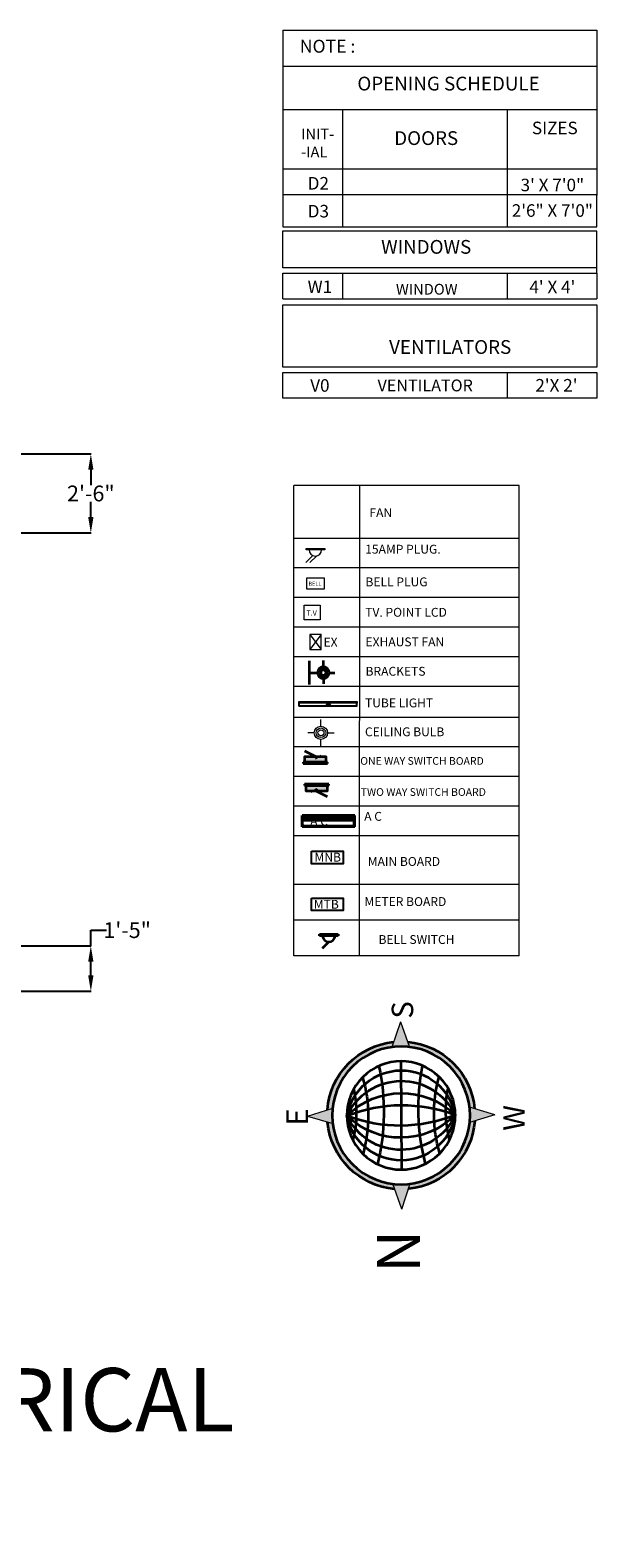
# Model space of a CAD drawing. Units: inches. Extents: x 329 to 1300, y 173 to 760.
# Tile 3 of 3: x 1085 to 1300, y 173 to 746. Entities that reach past the tile are written whole.
import ezdxf

# ---------------------------------------------------------------- set-up
doc = ezdxf.new("R2010")
doc.units = ezdxf.units.IN
doc.header["$MEASUREMENT"] = 0
doc.linetypes.add('HIDDEN', pattern=[0.375, 0.25, -0.125])
for name, color, linetype, lineweight in [('A -Elec', 6, 'Continuous', 18), ('A- WALL', 7, 'Continuous', 35), ('A-ANNO-SCHD', 80, 'Continuous', 13), ('A-ANNO-SCHD-HIDN', 80, 'HIDDEN', 13), ('A-ANNO-SYMB', 7, 'Continuous', 18), ('A-ANNO-TITL', 1, 'Continuous', 25), ('A-TEXT', 7, 'Continuous', 9), ('DIM', 7, 'Continuous', 9), ('DIMENSION', 80, 'Continuous', 13), ('E-ANNO-LEGD', 7, 'Continuous', 13), ('E-COMM', 1, 'Continuous', 18), ('E-EQPM-FANS', 1, 'Continuous', 18), ('E-LITE', 6, 'Continuous', 18), ('E-LITE-SWCH', 1, 'Continuous', 18), ('E-POWR-DEVC', 1, 'Continuous', 18), ('E-POWR-PANL', 1, 'Continuous', 25), ('Elec', 1, 'Continuous', 35), ('M-HVAC-EQPM', 1, 'Continuous', 18)]:
    doc.layers.add(name, color=color, linetype=linetype, lineweight=lineweight)
doc.styles.get("Standard").update_dxf_attribs({"font": 'arial.ttf'})
doc.dimstyles.get("Standard").update_dxf_attribs({"dimtxt": 6, "dimasz": 6, "dimexe": 0.18, "dimexo": 0.0625, "dimgap": 0.09, "dimtad": 0, "dimtih": 1, "dimtoh": 1, "dimdec": 1, "dimzin": 0, "dimdsep": 46, "dimlunit": 3, "dimtxsty": 'Standard', "dimcen": 0.09, "dimadec": 0, "dimazin": 0, "dimtfac": 1, "dimtdec": 1, "dimtofl": 0, "dimtmove": 0, "dimatfit": 3, "dimfxl": 1, "dimtolj": 1, "dimtzin": 0, "dimarcsym": 0})

# ---------------------------------------------------------------- blocks, each defined once
blk = doc.blocks.new('BELL SWITCH')
at = {"layer": 'Elec'}
for p, q in [((4981.810695824261, 3401.308516663301), (4981.810695824261, 3402.267205949833)), ((4981.810695824261, 3402.267205949833), (4993.567325880143, 3402.267205949833)), ((4993.567325880143, 3401.308516663301), (4981.810695824261, 3401.308516663301)), ((4987.689010852202, 3397.361748155474), (4983.521874140887, 3393.30038126191)), ((4993.567325880143, 3402.267205949833), (4993.567325880143, 3401.308516663301))]:
    blk.add_line(p, q, dxfattribs=at)
blk.add_arc((4987.689010852202, 3401.308516663301), 3.946768507828181, 180, 0, dxfattribs=at)
blk = doc.blocks.new('splight')
at = {"layer": 'Elec'}
for p, q in [((4618.165493646445, 527.1595508907546), (4627.57380882646, 527.1595508907546)), ((4622.869651236451, 527.1595508907546), (4622.869651236451, 523.8688723625129)), ((4620.576181531769, 521.5754026578305), (4618.052205676129, 521.5754026578305)), ((4622.869651236451, 519.2819329531479), (4622.869651236451, 517.0346704452847)), ((4625.163120941137, 521.5754026578305), (4627.232633020232, 521.5754026578305))]:
    blk.add_line(p, q, dxfattribs=at)
for radius in [2.293469704682637, 1.668469704682639, 1.043469704682639]:
    blk.add_circle((4622.869651236451, 521.5754026578305), radius, dxfattribs=at)
blk = doc.blocks.new('CIELING')
at = {"layer": 'A -Elec'}
for p, q in [((1070.869500591183, -8395.655580837194), (1070.869500591183, -8391.485789029257)), ((1066.613971407157, -8399.911110021205), (1062.44417959922, -8399.911110021205)), ((1070.869500591183, -8408.33643101315), (1070.869500591183, -8404.166639205214)), ((1075.125029775208, -8399.911110021205), (1079.294821583145, -8399.911110021205))]:
    blk.add_line(p, q, dxfattribs=at)
for radius in [4.255529184009533, 3.095842734009534, 1.936156284009533]:
    blk.add_circle((1070.869500591183, -8399.911110021205), radius, dxfattribs=at)
blk = doc.blocks.new('tube')
at = {"layer": 'A -Elec'}
for p, q in [((4592.607752765609, 556.7543292074987), (4641.607752765609, 556.7543292074987)), ((4592.607752765609, 555.2543292074988), (4592.607752765609, 556.7543292074987)), ((4593.107752765609, 555.2543292074988), (4593.107752765609, 556.7543292074987)), ((4593.107752765609, 556.3299144522243), (4593.407752765609, 556.3299144522243)), ((4593.107752765609, 556.2104979518087), (4593.407752765609, 556.2104979518087)), ((4593.107752765609, 555.8060867251079), (4593.407752765609, 555.8060867251079)), ((4593.107752765609, 555.6866702246923), (4593.407752765609, 555.6866702246923)), ((4593.407752765609, 555.2543292074988), (4593.407752765609, 556.7543292074987)), ((4593.407752765609, 556.5043292074988), (4640.807752765609, 556.5043292074988)), ((4593.407752765609, 556.2543292074987), (4640.807752765609, 556.2543292074987)), ((4593.407752765609, 556.0043292074988), (4640.807752765609, 556.0043292074988)), ((4593.407752765609, 555.7543292074988), (4640.807752765609, 555.7543292074988)), ((4593.407752765609, 555.5043292074988), (4640.807752765609, 555.5043292074988)), ((4640.807752765609, 555.2543292074988), (4640.807752765609, 556.7543292074987)), ((4640.807752765609, 556.3299144522243), (4641.107752765608, 556.3299144522243)), ((4640.807752765609, 556.2104979518087), (4641.107752765608, 556.2104979518087)), ((4640.807752765609, 555.8060867251079), (4641.107752765608, 555.8060867251079)), ((4640.807752765609, 555.6866702246923), (4641.107752765608, 555.6866702246923)), ((4641.107752765608, 556.7543292074987), (4641.107752765608, 555.2543292074988)), ((4641.107752765608, 555.2543292074988), (4641.107752765608, 556.7543292074987)), ((4641.607752765609, 556.7543292074987), (4641.607752765609, 555.2543292074988)), ((4592.607752765609, 552.7543292074987), (4592.607752765609, 555.2543292074988)), ((4592.607752765609, 552.7543292074987), (4641.607752765609, 552.7543292074987)), ((4641.107752765608, 555.2543292074988), (4593.107752765609, 555.2543292074988)), ((4593.107752765609, 555.2543292074988), (4593.107752765609, 553.2543292074988)), ((4593.107752765609, 553.2543292074988), (4593.107752765609, 555.2543292074988)), ((4593.107752765609, 553.2543292074988), (4641.607752765609, 553.2543292074988)), ((4641.107752765608, 553.2543292074988), (4641.107752765608, 555.2543292074988)), ((4641.607752765609, 552.7543292074987), (4641.607752765609, 555.2543292074988))]:
    blk.add_line(p, q, dxfattribs=at)
for points in [[(4615.603450108063, 553.2543292074988), (4619.112055423154, 553.2543292074988), (4619.112055423154, 554.3062122222327), (4615.603450108063, 554.3062122222327)], [(4619.112055423154, 553.7802707148657), (4619.112055423154, 553.7802707148657), (4619.112055423154, 553.7802707148657), (4619.112055423154, 553.7802707148657)], [(4619.112055423154, 553.7802707148657), (4619.813791770798, 553.7802707148657), (4619.813791770798, 553.2543292074988), (4619.112055423154, 553.2543292074988)]]:
    blk.add_lwpolyline(points, close=True, dxfattribs=at)
blk = doc.blocks.new('ac')
at = {"layer": 'Elec'}
for p, q in [((12718.33512872629, -53.78451556294852), (12674.35721837807, -53.78451556294852)), ((12674.35721837806, -63.01930683579224), (12674.35721837807, -53.78451556294852)), ((12674.88506837807, -57.52248662285011), (12717.80727872628, -57.52248662285011)), ((12675.81311487755, -57.52248662285011), (12675.81311487755, -53.78451556294851)), ((12717.02869991749, -54.85019267976269), (12675.81311487755, -54.85019267976269)), ((12717.02869991749, -56.20859049643797), (12675.81311487755, -56.20859049643797)), ((12717.02869991748, -57.52248662285011), (12717.02869991749, -53.78451556294851)), ((12718.33512872629, -63.01930683579224), (12718.33512872629, -53.78451556294852)), ((12718.33512872629, -63.01930683579224), (12674.35721837806, -63.01930683579224))]:
    blk.add_line(p, q, dxfattribs=at)
at = {"layer": 'Elec', "ltscale": 0.1}
for p, q in [((12674.88506837807, -61.49145683579366), (12674.88506837807, -53.78451556294851)), ((12717.02869991749, -54.35872395628861), (12675.81311487755, -54.35872395628861)), ((12717.02869991749, -55.65507023101156), (12675.81311487755, -55.65507023101157)), ((12717.02869991749, -56.84485043173038), (12675.81311487755, -56.84485043173037)), ((12716.80727872628, -62.49145683579365), (12675.88506837807, -62.49145683579365)), ((12717.80727872628, -61.49145683579366), (12717.80727872628, -53.78451556294851))]:
    blk.add_line(p, q, dxfattribs=at)
at = {"layer": 'Elec'}
for centre, start, end in [((12675.88506837807, -61.49145683579366), 180, 270), ((12716.80727872628, -61.49145683579366), 270, 0)]:
    blk.add_arc(centre, 1, start, end, dxfattribs=at)
blk = doc.blocks.new('DIRECTION')
at = {"layer": 'DIM', "ltscale": 35}
h = blk.add_hatch(color=256, dxfattribs=at)
h.dxf.hatch_style = 1
edge = h.paths.add_edge_path()
edge.add_line((2597.24832190935, 2408.269559539512), (2601.856533232682, 2393.62299110183))
edge.add_ellipse((2597.639423319343, 2353.481842285464), major_axis=(28.54028595385228, -28.5402859538523), ratio=0.9999999999827393, start_angle=129.0026750704451, end_angle=135.4089982327699)
edge.add_ellipse((2597.639423319602, 2353.481842285464), major_axis=(-28.54028595291803, -28.54028595291801), ratio=0.999999999985297, start_angle=225.4089982331304, end_angle=231.8159173823239)
edge.add_line((2592.849261358955, 2393.558645959323), (2597.248321909339, 2408.269559539583))
h = blk.add_hatch(color=256, dxfattribs=at)
h.dxf.hatch_style = 1
edge = h.paths.add_edge_path()
edge.add_line((2637.716337406115, 2348.692604170624), (2640.725786551334, 2349.752367405582))
edge.add_ellipse((2597.639423319343, 2353.481842285464), major_axis=(-30.58057945317442, -30.5805794531744), ratio=0.9999999999976388, start_angle=50.166226554127775, end_angle=130.0529151095595, ccw=False)
edge.add_line((2601.533664809112, 2310.41005845266), (2602.42916840349, 2313.404988786752))
edge.add_ellipse((2597.639423319343, 2353.481842285464), major_axis=(-28.54028595136435, -28.54028595136432), ratio=0.9999999999994514, start_angle=51.81532139532596, end_angle=128.185403391547)
edge = h.paths.add_edge_path()
edge.add_line((2593.421895860988, 2313.340737337358), (2594.360152675466, 2310.358877830749))
edge.add_ellipse((2597.639423319343, 2353.481842285464), major_axis=(-30.58057945314276, -30.58057945314273), ratio=0.9999999999967295, start_angle=320.7650813562228, end_angle=400.6513322142664, ccw=False)
edge.add_line((2554.610693956437, 2349.137635932355), (2557.634965847779, 2348.12094433685))
edge.add_ellipse((2597.639423319343, 2353.481842285464), major_axis=(28.54028595137265, -28.54028595137269), ratio=0.9999999999998977, start_angle=232.6325930742551, end_angle=309.0020790836279)
edge = h.paths.add_edge_path()
edge.add_line((2557.562509232831, 2358.271080400352), (2554.553060087694, 2357.211317165394))
edge.add_ellipse((2597.639423319343, 2353.481842285464), major_axis=(-30.58057945310715, -30.58057945310715), ratio=0.9999999999999497, start_angle=230.1666642515818, end_angle=310.0529151095499, ccw=False)
edge.add_line((2593.744852793148, 2396.553596367937), (2592.849261358943, 2393.558645959394))
edge.add_ellipse((2597.639423319343, 2353.481842285464), major_axis=(28.5402859513619, -28.54028595136188), ratio=0.9999999999987931, start_angle=141.8159173820852, end_angle=218.1854033915469)
edge = h.paths.add_edge_path()
edge.add_line((2601.85653323267, 2393.622991101876), (2600.918364535997, 2396.604831790109))
edge.add_ellipse((2597.639423319343, 2353.481842285464), major_axis=(-30.58057945312165, -30.58057945312163), ratio=0.9999999999985156, start_angle=140.765081356223, end_angle=220.6517699116423, ccw=False)
edge.add_line((2640.668152682508, 2357.826048638621), (2637.643880791167, 2358.842740234127))
edge.add_ellipse((2597.639423319343, 2353.481842285464), major_axis=(28.54028595137743, -28.54028595137745), ratio=0.9999999999999049, start_angle=52.63259307425506, end_angle=129.0026750705646)
h = blk.add_hatch(color=256, dxfattribs=at)
h.dxf.hatch_style = 1
edge = h.paths.add_edge_path()
edge.add_ellipse((2597.639423319343, 2353.481842285464), major_axis=(-28.54028595210723, -28.54028595210721), ratio=0.999999999994473, start_angle=308.1854033915466, end_angle=322.6325930742547)
edge.add_line((2557.634965847779, 2348.120944336826), (2542.851706063651, 2353.090740875343))
edge.add_line((2542.851706063651, 2353.090740875343), (2557.562509232831, 2358.271080400328))
h = blk.add_hatch(color=256, dxfattribs=at)
h.dxf.hatch_style = 1
edge = h.paths.add_edge_path()
edge.add_line((2637.643880791167, 2358.84274023415), (2652.427140575295, 2353.87294369554))
edge.add_line((2652.427140575295, 2353.87294369554), (2637.716337406114, 2348.692604170648))
edge.add_ellipse((2597.639423319343, 2353.481842285464), major_axis=(-28.54028595030189, -28.54028595030183), ratio=0.9999999999925798, start_angle=128.1854033915468, end_angle=142.632593074255)
h = blk.add_hatch(color=256, dxfattribs=at)
h.dxf.hatch_style = 1
edge = h.paths.add_edge_path()
edge.add_line((2602.42916840349, 2313.404988786869), (2598.030524729594, 2298.694125031464))
edge.add_line((2598.030524729594, 2298.69412503137), (2593.421895860988, 2313.340737337334))
edge.add_ellipse((2597.639423319602, 2353.481842285464), major_axis=(28.54028595190623, -28.54028595190623), ratio=0.9999999999939888, start_angle=-50.99792091661058, end_angle=-44.59100176735014)
edge.add_ellipse((2597.639423319343, 2353.481842285464), major_axis=(-28.54028595335771, -28.54028595335769), ratio=0.9999999999832972, start_angle=45.40899823301023, end_angle=51.81532139544526)
at = {"layer": 'A- WALL', "ltscale": 35}
blk.add_line((2629.34444276032, 2353.708168156072), (2565.934403878626, 2353.255516414717), dxfattribs=at)
at = {"layer": 'A- WALL', "ltscale": 35, "extrusion": (0, 0, -1)}
for centre, major_axis, ratio, start_param, end_param in [((2597.639423319343, 2353.481842285418), (-30.58057945312132, -30.58057945312131), 0.9999999999987959, 0.8717410831091346, 2.266019187658509), ((2597.639423319343, 2353.481842285418), (28.5402859514277, -28.5402859514277), 0.9999999999973692, 3.919852451189786, 10.20303775836937), ((2597.639423319343, 2353.481842285418), (-30.58057945314268, -30.58057945314266), 0.9999999999988618, 2.432085421867908, 3.826371165679486), ((2597.639423319343, 2353.481842285418), (22.41940544614458, -22.41940544614459), 0.999999999999132, 3.919852451188904, 10.20303775836849), ((2603.542187591361, 2353.523989522555), (22.80466912504525, -22.80466912504527), 0.9999999999934116, 0.9623333078138184, 3.735775406983438), ((2612.505423052941, 2353.587989301701), (-24.76160024723522, -24.76160024723521), 0.9999999999992525, -0.3540869259178678, 1.910602987118144), ((2629.757673802409, 2353.71112763613), (-31.9131967420592, -31.91319674205919), 0.9999999999985343, -0.0006610730671919, 1.55718066820378), ((2678.031679859687, 2354.055802032412), (-61.10857846222063, -61.10857846222057), 0.999999999998412, 0.4026080436482158, 1.153909784551204), ((2517.246998575127, 2352.907900606915), (61.1085784622124, -61.10857846221246), 0.9999999999999429, 5.114997024032398, 5.866298764935286), ((2565.521005037576, 2353.252518252051), (-31.91319674206676, -31.91319674206674), 0.9999999999991755, 3.140929813589933, 4.698771554849301), ((2591.736490906592, 2353.439704278876), (-22.80466912498845, -22.80466912498845), 0.9999999999995747, 2.533131401603469, 5.306573500773075), ((2582.773255331945, 2353.375720337799), (-24.76160024727029, -24.76160024727029), 0.9999999999990459, 2.78750749467719, 5.052197407698938), ((2597.115156409695, 2454.394147896003), (-57.71452300102988, -57.71452300102983), 0.9999999999994852, -1.068719002289636, -0.5124677756952505), ((2599.782951195766, 2490.828885281749), (89.95633825820524, -89.95633825820524), 0.9999999999996148, 0.5732801118446276, 1.028726990569549), ((2597.639423319343, 2353.481842285418), (-30.58057945309982, -30.5805794530998), 0.9999999999997768, -0.7094995924610965, 0.6847785120890495), ((2597.639423319343, 2353.481842285418), (-30.58057945319512, -30.58057945319512), 0.9999999999962719, 4.013333736700001, 5.407619480506816), ((2601.743533004009, 2216.179397968859), (-89.95633825845869, -89.95633825845869), 0.9999999999989515, 2.098588931419211, 2.554035810148795), ((2600.498417980858, 2261.332926481243), (-46.62855256648622, -46.6285525664862), 0.9999999999990784, 2.096633230266009, 2.553724030937174)]:
    blk.add_ellipse(centre, major_axis=major_axis, ratio=ratio, start_param=start_param, end_param=end_param, dxfattribs=at)
at = {"layer": 'A- WALL', "ltscale": 35, "extrusion": (0, 0, -0.9999999999999998)}
for centre, major_axis, ratio, start_param, end_param in [((2599.182585971628, 2445.662182832683), (46.62855256632114, -46.62855256632116), 0.9999999999994293, 0.5735918910566035, 1.030682691728694), ((2598.555858798734, 2252.572336165166), (-57.71452300096218, -57.71452300096211), 0.9999999999999362, 2.068987370893696, 2.625238597487658)]:
    blk.add_ellipse(centre, major_axis=major_axis, ratio=ratio, start_param=start_param, end_param=end_param, dxfattribs=at)
at = {"layer": 'DIM', "ltscale": 35}
for p, q in [((2597.24832190935, 2408.269559539489), (2592.827539238222, 2393.486004940269)), ((2597.24832190935, 2408.269559539489), (2601.879338537261, 2393.550507565663)), ((2542.851706063651, 2353.090740875319), (2557.656003696302, 2358.30400403195)), ((2652.427140575295, 2353.872943695493), (2637.549925830003, 2358.874325760384)), ((2542.851706063651, 2353.090740875319), (2557.728920809025, 2348.089358810546)), ((2652.427140575295, 2353.872943695493), (2637.622842942642, 2348.659680538956)), ((2598.030524729594, 2298.694125031323), (2593.399138912629, 2313.41306084311)), ((2598.030524729594, 2298.694125031323), (2602.450936591041, 2313.477790510296))]:
    blk.add_line(p, q, dxfattribs=at)
at = {"layer": 'A-TEXT', "char_height": 13.629465702112, "width": 273.2349075094469, "attachment_point": 2}
for s, insert in [('{\\fTimes New Roman|b0|i0|c0|p18;\\H0.9233x;E}', (2596.77738151443, 2420.65579489876)), ('{\\fTimes New Roman|b0|i0|c0|p18;\\H0.9233x;S}', (2659.361945474433, 2358.999040747372)), ('{\\fTimes New Roman|b0|i0|c0|p18;\\H0.9233x;W}', (2596.170612003199, 2293.619718441945))]:
    blk.add_mtext(s, dxfattribs=dict(at, insert=insert))
at = {"layer": 'A-TEXT', "insert": (2518.058106811495, 2342.398918831673), "char_height": 27.25893140422401, "width": 546.4698150188938, "attachment_point": 2, "rotation": 179.99999999999997}
blk.add_mtext('{\\fTimes New Roman|b0|i0|c0|p18;\\H0.9233x;N}', dxfattribs=at)
blk = doc.blocks.new('elec box')
at = {"layer": 'Elec'}
blk.add_hatch(color=256, dxfattribs=at).paths.add_polyline_path([(3828.234962737587, 599.2881263179643), (3828.234962737587, 594.7881263179643), (3844.734962737589, 594.7881263179643), (3844.734962737589, 599.2881263179643)])
for p, q in [((3836.484962737588, 599.2881263179643), (3828.066979685118, 603.4529863194257)), ((3846.10280273742, 594.7881263179643), (3826.830962060027, 594.7881263179643)), ((3826.830962060027, 594.7881263179643), (3826.830962060027, 593.8893551118417)), ((3826.830962060027, 593.8893551118417), (3846.10280273742, 593.8893551118417)), ((3846.10280273742, 593.8893551118417), (3846.10280273742, 594.7881263179643))]:
    blk.add_line(p, q, dxfattribs=at)
blk.add_lwpolyline([(3828.234962737587, 594.7881263179643), (3828.234962737587, 599.2881263179643), (3844.734962737589, 599.2881263179643), (3844.734962737589, 594.7881263179643), (3828.234962737587, 594.7881263179643)], dxfattribs=at)
blk = doc.blocks.new('SWITCHBOARD-1WAY')
blk.add_line((4.634819752865951, 1.728879398226013), (6.643515217023832, 3.124148960297475))
at = {"xscale": 0.480395109260985, "yscale": 0.480395109260985, "zscale": 0.480395109260985}
blk.add_blockref('elec box', (-1838.390897871826, -285.3016910940941), dxfattribs=at)
blk = doc.blocks.new('SWITCHBOARD-2WAY')
for p, q in [((4.622940541207071, 2.865345524835674), (2.614245077048735, 1.470075962730788)), ((4.62294053581013, 2.865345524868871), (6.622245607648665, 1.456653277292389))]:
    blk.add_line(p, q)
at = {"xscale": 0.480395109260985, "yscale": 0.480395109260985, "zscale": 0.480395109260985, "rotation": 180}
blk.add_blockref('elec box', (1847.648658163208, 289.8959160171557), dxfattribs=at)
blk = doc.blocks.new('BOARD-MAIN')
blk.add_lwpolyline([(-0.0002187870763919, 4.703149366078037), (12.06213643445835, 4.703149366078037), (12.06213643445835, 0.0003459323467041), (-0.0002187870763919, 0.0003459323467041)], close=True)
blk.add_text('MNB', height=3.362765764821897).set_placement((1.143365574901963, 0.7969912451682148))
blk = doc.blocks.new('BOARD-METER')
blk.add_lwpolyline([(-0.0002187870763919, 4.702370896325646), (12.06213643445835, 4.702370896325646), (12.06213643445835, -0.0004325374056862), (-0.0002187870763919, -0.0004325374056862)], close=True)
blk.add_text('MTB', height=3.362765764821897).set_placement((0.872471072623739, 0.6935034008668027))
blk = doc.blocks.new('BELL-POINT')
blk.add_lwpolyline([(0.0003646803647825, 4.272259619429178), (6.557693859329447, 4.272259619429178), (6.557693859329447, -0.0002068059475278), (0.0003646803647825, -0.0002068059475278)], close=True)
at = {"insert": (0.6443699543428921, 2.798315981574205), "char_height": 1.537264349632867, "attachment_point": 1}
blk.add_mtext('BELL', dxfattribs=at)
blk = doc.blocks.new('TV-POINT')
blk.add_lwpolyline([(0.0003473057104202, 5.568134957917663), (6.101081488943691, 5.568134957917663), (6.101081488943691, -5.40124440249e-05), (0.0003473057104202, -5.40124440249e-05)], close=True)
at = {"transparency": 33554676}
blk.add_lwpolyline([(0.0003473057104202, 5.568134957917663), (6.101081488943691, 5.568134957917663), (6.101081488943691, -5.40124440249e-05), (0.0003473057104202, -5.40124440249e-05)], close=True, dxfattribs=at)
at = {"insert": (0.839661815510226, 3.647184413183822), "char_height": 2.003474701485161, "attachment_point": 1}
blk.add_mtext('T.V ', dxfattribs=at)
at = {"transparency": 33554676, "insert": (0.839661815510226, 3.647184413183822), "char_height": 2.003474701485161, "attachment_point": 1}
blk.add_mtext('T.V ', dxfattribs=at)
blk = doc.blocks.new('*D53')
at = {"layer": 'Defpoints', "color": 0, "transparency": 16777216}
for p in [(1072.975195, 397.8396700000002), (1107.825195000001, 397.8396700000002), (1072.975195, 380.6172230000001)]:
    blk.add_point(p, dxfattribs=at)
at = {"layer": 'DIMENSION', "color": 0, "lineweight": -2, "transparency": 16777216}
for p, q in [((1107.825195000001, 397.8396700000002), (1107.825195000001, 403.8396700000002)), ((1107.825195000001, 403.8396700000002), (1113.825195000001, 403.8396700000002)), ((1073.037695, 397.8396700000002), (1108.005195000001, 397.8396700000002)), ((1107.825195000001, 386.6172230000002), (1107.825195000001, 391.8396700000002)), ((1073.037695, 380.6172230000001), (1108.005195000001, 380.6172230000001))]:
    blk.add_line(p, q, dxfattribs=at)
at = {"layer": 'DIMENSION', "color": 0, "transparency": 16777216}
for points in [[(1106.825195, 391.8396700000002), (1108.825195000001, 391.8396700000002), (1107.825195000001, 397.8396700000002)], [(1106.825195, 386.6172230000002), (1108.825195000001, 386.6172230000002), (1107.825195000001, 380.6172230000001)]]:
    blk.add_solid(points, dxfattribs=at)
at = {"layer": 'DIMENSION', "color": 0, "transparency": 16777216, "insert": (1121.607555163711, 403.8396699999998), "char_height": 6, "attachment_point": 5}
blk.add_mtext('\\A1;1\'-5"', dxfattribs=at)
blk = doc.blocks.new('*D58')
at = {"layer": 'Defpoints', "color": 0, "transparency": 16777216}
for p in [(1072.975195, 584.6172230000002), (1107.825195000001, 584.6172230000002), (1072.975195, 554.6176680000002)]:
    blk.add_point(p, dxfattribs=at)
at = {"layer": 'DIMENSION', "color": 0, "lineweight": -2, "transparency": 16777216}
for p, q in [((1073.037695, 584.6172230000002), (1108.005195000001, 584.6172230000002)), ((1107.825195000001, 578.6172230000001), (1107.825195000001, 572.7708834263303)), ((1107.825195000001, 560.6176680000002), (1107.825195000001, 566.4640075736698)), ((1073.037695, 554.6176680000002), (1108.005195000001, 554.6176680000002))]:
    blk.add_line(p, q, dxfattribs=at)
at = {"layer": 'DIMENSION', "color": 0, "transparency": 16777216}
for points in [[(1106.825195, 578.6172230000001), (1108.825195000001, 578.6172230000001), (1107.825195000001, 584.6172230000002)], [(1106.825195, 560.6176680000002), (1108.825195000001, 560.6176680000002), (1107.825195000001, 554.6176680000002)]]:
    blk.add_solid(points, dxfattribs=at)
at = {"layer": 'DIMENSION', "color": 0, "transparency": 16777216, "insert": (1107.825195000001, 569.6174454999996), "char_height": 6, "attachment_point": 5}
blk.add_mtext('\\A1;2\'-6"', dxfattribs=at)

msp = doc.modelspace()

# ---------------------------------------------------------------- linework, layer by layer
at = {"layer": 'A-ANNO-SCHD'}
for p, q in [((1180.764631489147, 745.5055112249477), (1180.764631489148, 692.8007288449498)), ((1180.764631489245, 731.79337437694), (1300.019283235984, 731.79337437694)), ((1180.764631489147, 715.3419340972092), (1300.019283183399, 715.3419340972092)), ((1203.545971529147, 692.8007288449497), (1203.545971529147, 715.3419340972092)), ((1266.081536151576, 692.8007288449497), (1266.081536151576, 715.3419340972092)), ((1180.764631489147, 692.8007288449497), (1300.019283111212, 692.8007288449497)), ((1180.764631602208, 692.8007288449497), (1300.019283193337, 692.8007288449497)), ((1180.764631602208, 692.8007288449497), (1180.764631602208, 683.0965949914959)), ((1203.545971642209, 670.8103882662031), (1203.545971642209, 692.8007288449497)), ((1266.081536264637, 670.8103882662031), (1266.081536264637, 692.8007288449497)), ((1180.764631602208, 683.0965949914959), (1300.019283162303, 683.0965949914959)), ((1180.764631602208, 683.0965949914959), (1180.764631602208, 670.8103882662031)), ((1300.019283162303, 670.8103882662031), (1300.019283203989, 682.7813817655821)), ((1180.764631602208, 670.8103882662031), (1300.019283162303, 670.8103882662031)), ((1180.797553005946, 643.4874799432256), (1180.797553005946, 653.1916137966792)), ((1203.570807377725, 643.4874799432256), (1203.578893045945, 653.1916137966792)), ((1266.081536493868, 643.4874799432256), (1266.081536493868, 653.1916137966792)), ((1180.79755199479, 641.2766888593371), (1300.052202274381, 641.2766888593371)), ((1180.797553005946, 643.4874799432256), (1300.052203285506, 643.4874799432256)), ((1266.114456832746, 605.7706758156932), (1266.114456832746, 615.4748096691474))]:
    msp.add_line(p, q, dxfattribs=at)
for points in [[(1180.764631489147, 745.5055112249477), (1300.019283466991, 745.5055112249477), (1300.019283193337, 692.8007288449497)], [(1300.019283256012, 692.8007288449497), (1300.019283203989, 682.7813817655821)], [(1300.019283184774, 655.2480771217535), (1180.764631831538, 655.2480771217535), (1180.764631831538, 669.3426249146187), (1300.019283229802, 669.3426249146187)], [(1180.764631831538, 653.1916137966792), (1300.019283178177, 653.1916137966792), (1300.019283148748, 643.4874799432256)], [(1300.052203195611, 605.7706758156932), (1180.797552170193, 605.7706758156932), (1180.797552170193, 615.4748096691474), (1300.052203257582, 615.4748096691474)], [(1300.052203257582, 615.4748096691474), (1300.052203195513, 605.7706758156932), (1183.020751431793, 605.7706758156932)]]:
    msp.add_lwpolyline(points, dxfattribs=at)
msp.add_lwpolyline([(1300.052203264178, 617.5312729942215), (1180.797552170193, 617.5312729942215), (1180.797552139257, 641.2766888593371), (1300.052203285506, 641.2766888593371), (1300.052203264178, 617.5312729942215)], close=True, dxfattribs=at)
at = {"layer": 'A-ANNO-SCHD-HIDN'}
msp.add_line((1300.019283178177, 653.1916137966792), (1300.019283229802, 669.3426249146187), dxfattribs=at)
at = {"layer": 'E-ANNO-LEGD'}
for p, q in [((1184.959654740691, 394.1126091913483), (1184.959654740691, 572.6625877864531)), ((1270.543659946572, 572.6625877864531), (1184.959654740691, 572.6625877864531)), ((1209.937679575464, 572.6625877864531), (1209.794773566678, 394.1126091913483)), ((1270.543659946564, 394.1126091913483), (1270.543659946564, 572.6625877864531)), ((1270.543659946572, 552.5776421528295), (1184.959654740691, 552.5776421528295)), ((1270.543659946572, 552.5776421528461), (1184.959654740691, 552.5776421528461)), ((1270.543659946572, 541.3193157995508), (1184.959654740691, 541.3193157995508)), ((1270.543659946564, 530.0609894462724), (1184.959654740674, 530.0609894462724)), ((1270.543659946572, 518.8026630929772), (1184.959654740691, 518.8026630929772)), ((1270.543659946572, 507.5443367396989), (1184.959654740691, 507.5443367396989)), ((1270.543659946572, 496.2860103864203), (1184.959654740691, 496.2860103864203)), ((1270.543659946564, 484.620219712683), (1184.959654740674, 484.620219712683)), ((1270.543659946564, 473.3618933593878), (1184.959654740674, 473.3618933593878)), ((1270.543659946564, 462.1035670061092), (1184.959654740674, 462.1035670061092)), ((1270.543659946572, 450.8452406528143), (1184.959654740691, 450.8452406528143)), ((1270.543659946572, 439.5869142995358), (1184.959654740691, 439.5869142995358)), ((1270.543659946572, 421.1845245302782), (1184.959654740691, 421.1845245302782)), ((1270.543659946572, 407.6485668608214), (1184.959654740691, 407.6485668608214)), ((1270.543659946572, 394.112609191348), (1184.959654740691, 394.112609191348))]:
    msp.add_line(p, q, dxfattribs=at)
at = {"layer": 'E-EQPM-FANS'}
for p, q in [((1190.972251278176, 516.080590054686), (1195.295807261518, 510.3158487435527)), ((1195.295807261518, 516.080590054686), (1190.972251278176, 510.3158487435527))]:
    msp.add_line(p, q, dxfattribs=at)
msp.add_lwpolyline([(1195.295807261518, 516.080590054686), (1190.972251278176, 516.080590054686), (1190.972251278176, 510.3158487435527), (1195.295807261518, 510.3158487435527)], close=True, dxfattribs=at)
at = {"layer": 'E-POWR-DEVC'}
for p, q in [((1192.192004056653, 546.0294076109836), (1189.489318438653, 543.3953212698858)), ((1189.6041370322, 548.7798446770012), (1196.663921507486, 548.7798446770012)), ((1189.6041370322, 548.2041576213124), (1189.6041370322, 548.7798446770012)), ((1196.663921507486, 548.2041576213124), (1189.6041370322, 548.2041576213124)), ((1193.491037868239, 545.8341472606285), (1190.98869774856, 543.3953212698858)), ((1196.663921507486, 548.7798446770012), (1196.663921507486, 548.2041576213124))]:
    msp.add_line(p, q, dxfattribs=at)
msp.add_arc((1193.134029269855, 548.2041576213124), 2.370010360678894, 180, 0, dxfattribs=at)

# ---------------------------------------------------------------- block references
at = {"layer": 'A-ANNO-SYMB', "xscale": 0.648641096179051, "yscale": 0.648641096179051, "zscale": 0.648641096179051, "rotation": 89.99999999999999}
msp.add_blockref('DIRECTION', (2752.259646797853, -1351.44425865697), dxfattribs=at)
at = {"layer": 'E-COMM'}
for name, p in [('BELL-POINT', (1189.855, 533.3029999999999)), ('TV-POINT', (1188.873, 521.584))]:
    msp.add_blockref(name, p, dxfattribs=at)
at = {"layer": 'E-COMM', "xscale": 0.6004938865802444, "yscale": 0.6004938865802444, "zscale": 0.6004938865802444}
msp.add_blockref('BELL SWITCH', (-1796.82670387379, -1640.746660574752), dxfattribs=at)
at = {"layer": 'E-LITE', "xscale": -0.9617510087435096, "yscale": 0.9617510087435096, "zscale": 0.9617510087390623, "rotation": 89.99999999999976}
msp.add_blockref('splight', (1697.790221708665, 4947.627396269933), dxfattribs=at)
at = {"layer": 'E-LITE', "transparency": 33554676}
for name, p, xscale, yscale, zscale in [('tube', (-895.8039405541317, 238.1778628530538), 0.4534687213066354, 0.4534687213066354, 0.4534687213066354), ('CIELING', (560.1411184287304, 5460.334799110341), 0.5930528030907906, 0.5930528030907906, 0.5930528030907906)]:
    msp.add_blockref(name, p, dxfattribs=dict(at, xscale=xscale, yscale=yscale, zscale=zscale))
at = {"layer": 'E-LITE-SWCH'}
for name, p in [('SWITCHBOARD-1WAY', (1188.505, 467.154)), ('SWITCHBOARD-2WAY', (1188.97, 454.6109999999999))]:
    msp.add_blockref(name, p, dxfattribs=at)
at = {"layer": 'E-POWR-PANL'}
for name, p in [('BOARD-MAIN', (1191.663, 429.058)), ('BOARD-METER', (1191.663, 411.274))]:
    msp.add_blockref(name, p, dxfattribs=at)
at = {"layer": 'M-HVAC-EQPM', "xscale": 0.4550488862921059, "yscale": 0.4550488862921059, "zscale": 0.4550488862921059}
msp.add_blockref('ac', (-4579.394279337683, 471.7702579085111), dxfattribs=at)

# ---------------------------------------------------------------- texts
at = {"layer": 'A-ANNO-SCHD'}
for s, insert, char_height, width, attachment_point in [('{\\fTimes New Roman|b0|i0|c0|p18;NOTE :}', (1187.215938366661, 741.8534495594276), 4.902323584711946, 121.5202880819514, 1), ('{\\fTimes New Roman|b0|i0|c0|p18;OPENING SCHEDULE}', (1243.705288109431, 725.2184163915614), 5.229145157026076, 144.0307668520136, 5), ('{\\fTimes New Roman|b0|i0|c0|p18;\\H0.8x;SIZES}', (1284.076843480513, 710.7587232015904), 5.953076141217599, 38.19427163934395, 2), ('{\\fTimes New Roman|b0|i0|c0|p18;INIT-\\P-IAL}', (1187.713061204559, 708.1028402334518), 4.085269653926621, 14.45685851554141, 1), ('{\\fTimes New Roman|b0|i0|c0|p18;DOORS}', (1235.219548392662, 704.519553381341), 5.229145157026076, 144.0307668520136, 5), ('{\\fTimes New Roman|b0|i0|c0|p18;\\H0.8x;D2}', (1194.25027744195, 687.3697011401819), 5.953076141217599, 20.39887023007676, 5), ('{\\fTimes New Roman|b0|i0|c0|p18;\\H0.8x;3\' X 7\'0"}', (1283.149302506849, 686.7272215760432), 5.953092231351539, 47.33954989007876, 5), ('{\\fTimes New Roman|b0|i0|c0|p18;\\H0.8x;D3}', (1194.25027744195, 676.7820899671447), 5.953076141217599, 20.39887023007676, 5), ('{\\fTimes New Roman|b0|i0|c0|p18;\\H0.8x;2\'6" X 7\'0"}', (1283.149302506849, 677.0230877226069), 5.953092231351539, 47.33954989007876, 5), ('{\\fTimes New Roman|b0|i0|c0|p18;WINDOWS }', (1235.219548734954, 663.228342788128), 5.229145157026076, 144.0307668520136, 5), ('{\\fTimes New Roman|b0|i0|c0|p18;\\H0.8x;W1}', (1194.836548582878, 648.0770199451), 5.953092231351539, 20.39887023007676, 5), ('{\\fTimes New Roman|b0|i0|c0|p18; WINDOW}', (1234.813754213683, 647.1421674586248), 4.085269653926621, 80.50969521635155, 5), ("{\\fTimes New Roman|b0|i0|c0|p18;\\H0.8x;4' X 4'}", (1283.149302506849, 648.0085728507268), 5.953092231351539, 47.33954989007876, 5), ('{\\fTimes New Roman|b0|i0|c0|p18;VENTILATORS }', (1244.330101000106, 625.2168334710759), 5.229145157026076, 144.0307668520136, 5), ('{\\fTimes New Roman|b0|i0|c0|p18;\\H0.8x;V0}', (1194.836547747219, 610.6227427424069), 5.953076141217599, 20.39887023007676, 5), ('{\\fTimes New Roman|b0|i0|c0|p18;VENTILATOR}', (1234.8466745215, 610.6227427424069), 4.493796619319285, 80.50969521635155, 5), ("{\\fTimes New Roman|b0|i0|c0|p18;\\H0.8x;2'X 2'}", (1284.692262875335, 610.6800977262747), 5.953092231351539, 47.33954989007876, 5)]:
    msp.add_mtext(s, dxfattribs=dict(at, insert=insert, char_height=char_height, width=width, attachment_point=attachment_point))
at = {"layer": 'A-ANNO-TITL', "insert": (939.5434997474684, 237.5531046851913), "char_height": 24, "attachment_point": 2}
msp.add_mtext_dynamic_manual_height_columns('FURNITURE AND ELECTRICAL LAYOUT', width=477.7756710489011, gutter_width=169.0676303890764, heights=[150.7082665236336], dxfattribs=at)
at = {"layer": 'E-ANNO-LEGD'}
for s, height, p in [('FAN', 3.362765764821897, (1213.66135092405, 560.6421003971888)), ('15AMP PLUG.', 3.362765764821897, (1212.053085712437, 546.7691754886328)), ('BELL PLUG', 3.362765764821897, (1212.16026781614, 534.3577798045718)), ('TV. POINT LCD', 3.362765764821897, (1212.066284368528, 522.8180764400341)), ('EXHAUST FAN', 3.362765764821897, (1212.160042412129, 511.5801917224452)), ('BRACKETS', 3.362765764821897, (1212.176316580505, 500.4237773457606)), ('TUBE LIGHT', 3.362765764821897, (1211.972000382298, 488.4100685414174)), ('CEILING BULB', 3.362765764821897, (1211.968083361778, 477.4476625777198)), ('ONE WAY SWITCH BOARD', 2.913500258641691, (1210.174303839906, 466.6151066126531)), ('TWO WAY SWITCH BOARD', 2.913500258641691, (1210.338661156364, 454.8043479233633)), (' A C', 3.362765764821897, (1210.646417418708, 445.3505072351628)), ('MAIN BOARD', 3.362765764821897, (1213.026493357648, 428.2178846862608)), ('METER BOARD', 3.362765764821897, (1211.778237569376, 412.9911326219675)), ('BELL SWITCH', 3.362765764821897, (1217.119407639367, 398.5833108470402))]:
    msp.add_text(s, height=height, dxfattribs=at).set_placement(p)
at = {"layer": 'E-EQPM-FANS', "insert": (1196.221125005864, 514.8676388338451), "char_height": 3.362765764821897, "width": 5.871009998848781, "attachment_point": 1}
msp.add_mtext('EX', dxfattribs=at)
at = {"layer": 'M-HVAC-EQPM'}
msp.add_text(' A C', height=3.362765764821897, dxfattribs=at).set_placement((1190.118241273142, 443.5616576455603))

# ---------------------------------------------------------------- dimensions: what is measured, and where the dimension line sits
at = {"layer": 'DIMENSION'}
for base, p1, p2, picture, middle in [((1107.825195000001, 584.6172230000002), (1072.975195, 554.617668), (1072.975195, 584.6172229999999), '*D58', (1107.825195000001, 569.6174454999996)), ((1107.825195000001, 397.8396700000002), (1072.975195, 380.6172230000001), (1072.975195, 397.83967), '*D53', (1121.607555163711, 403.8396699999998))]:
    dim = msp.add_linear_dim(base=base, p1=p1, p2=p2, angle=90, dimstyle='Standard', override={"dimdec": 1, "dimlfac": 1, "dimrnd": 0, "dimzin": 1, "dimdsep": 46, "dimlunit": 4, "dimfrac": 2}, dxfattribs=at)
    dim.commit()
    dim.dimension.update_dxf_attribs({"geometry": picture, "text_midpoint": middle})

doc.saveas('drawing.dxf')
